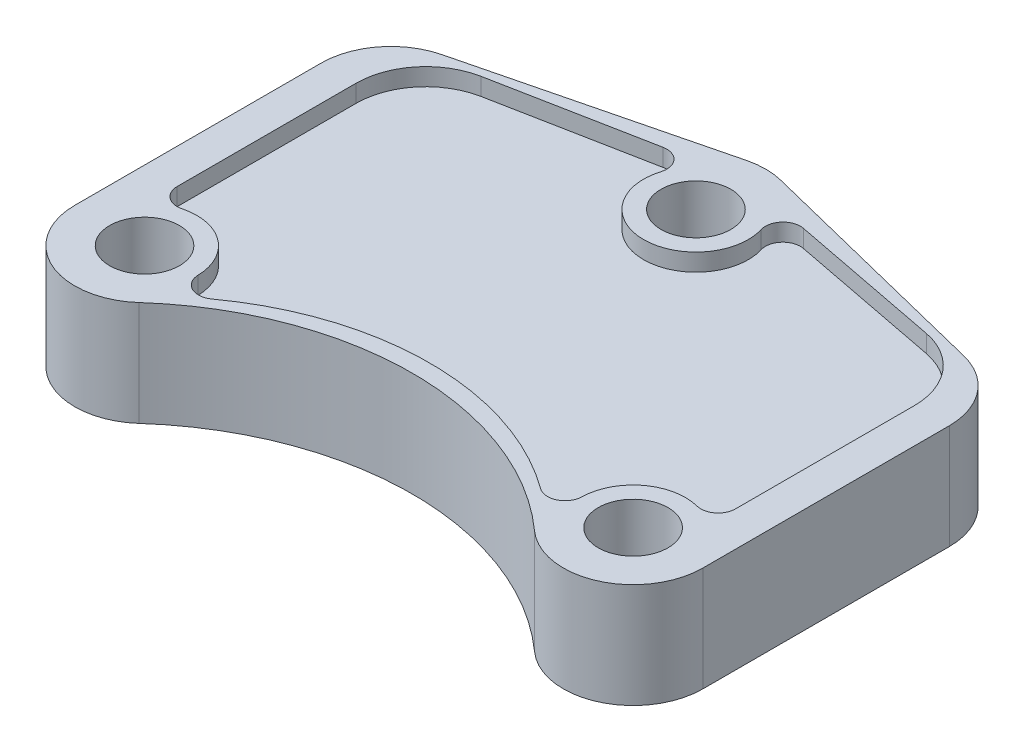
ISO-10303-21;
HEADER;
FILE_DESCRIPTION(('STEP AP214'),'2;1');
FILE_NAME('part.step','',(''),(''),'','','');
FILE_SCHEMA(('AUTOMOTIVE_DESIGN { 1 0 10303 214 1 1 1 1 }'));
ENDSEC;
DATA;
#1=APPLICATION_CONTEXT('core data for automotive mechanical design processes');
#2=APPLICATION_PROTOCOL_DEFINITION('international standard','automotive_design',2000,#1);
#3=PRODUCT_CONTEXT('',#1,'mechanical');
#4=PRODUCT('Part','Part','',(#3));
#5=PRODUCT_RELATED_PRODUCT_CATEGORY('part','',(#4));
#6=PRODUCT_DEFINITION_FORMATION('','',#4);
#7=PRODUCT_DEFINITION_CONTEXT('part definition',#1,'design');
#8=PRODUCT_DEFINITION('design','',#6,#7);
#9=PRODUCT_DEFINITION_SHAPE('','',#8);
#10=(LENGTH_UNIT() NAMED_UNIT(*) SI_UNIT(.MILLI.,.METRE.));
#11=(NAMED_UNIT(*) PLANE_ANGLE_UNIT() SI_UNIT($,.RADIAN.));
#12=(NAMED_UNIT(*) SI_UNIT($,.STERADIAN.) SOLID_ANGLE_UNIT());
#13=UNCERTAINTY_MEASURE_WITH_UNIT(LENGTH_MEASURE(1.E-05),#10,'distance_accuracy_value','');
#14=(GEOMETRIC_REPRESENTATION_CONTEXT(3) GLOBAL_UNCERTAINTY_ASSIGNED_CONTEXT((#13)) GLOBAL_UNIT_ASSIGNED_CONTEXT((#10,
#11,#12)) REPRESENTATION_CONTEXT('',''));
#15=CARTESIAN_POINT('',(0.,0.,0.));
#16=DIRECTION('',(0.,0.,1.));
#17=DIRECTION('',(1.,0.,0.));
#18=AXIS2_PLACEMENT_3D('',#15,#16,#17);
#19=CARTESIAN_POINT('',(-50.0055751114862,30.,87.5277994307735));
#20=DIRECTION('',(0.,-1.,0.));
#21=DIRECTION('',(0.,0.,-1.));
#22=AXIS2_PLACEMENT_3D('',#19,#20,#21);
#23=CYLINDRICAL_SURFACE('',#22,5.);
#24=DIRECTION('',(0.,-1.,0.));
#25=VECTOR('',#24,1.);
#26=CARTESIAN_POINT('',(-47.0640706931635,30.,91.5710100061687));
#27=LINE('',#26,#25);
#28=CARTESIAN_POINT('',(-47.0640706931635,30.,91.5710100061687));
#29=VERTEX_POINT('',#28);
#30=CARTESIAN_POINT('',(-47.0640706931635,25.,91.5710100061687));
#31=VERTEX_POINT('',#30);
#32=EDGE_CURVE('E268',#29,#31,#27,.T.);
#33=ORIENTED_EDGE('',*,*,#32,.T.);
#34=CARTESIAN_POINT('',(-50.0055751114862,25.,87.5277994307735));
#35=DIRECTION('',(0.,-1.,0.));
#36=DIRECTION('',(0.,0.,-1.));
#37=AXIS2_PLACEMENT_3D('',#34,#35,#36);
#38=CIRCLE('',#37,4.99999999999999);
#39=CARTESIAN_POINT('',(-55.0041813336146,25.,87.6458495730801));
#40=VERTEX_POINT('',#39);
#41=EDGE_CURVE('E740',#31,#40,#38,.T.);
#42=ORIENTED_EDGE('',*,*,#41,.T.);
#43=DIRECTION('',(0.,-1.,0.));
#44=VECTOR('',#43,1.);
#45=CARTESIAN_POINT('',(-55.0041813336146,30.,87.6458495730801));
#46=LINE('',#45,#44);
#47=CARTESIAN_POINT('',(-55.0041813336146,30.,87.6458495730801));
#48=VERTEX_POINT('',#47);
#49=EDGE_CURVE('E724',#48,#40,#46,.T.);
#50=ORIENTED_EDGE('',*,*,#49,.F.);
#51=CARTESIAN_POINT('',(-50.0055751114862,30.,87.5277994307735));
#52=DIRECTION('',(0.,1.,0.));
#53=DIRECTION('',(0.,0.,1.));
#54=AXIS2_PLACEMENT_3D('',#51,#52,#53);
#55=CIRCLE('',#54,5.);
#56=EDGE_CURVE('E731',#48,#29,#55,.T.);
#57=ORIENTED_EDGE('',*,*,#56,.T.);
#58=EDGE_LOOP('',(#33,#42,#50,#57));
#59=FACE_BOUND('',#58,.T.);
#60=ADVANCED_FACE('F39',(#59),#23,.F.);
#61=CARTESIAN_POINT('',(0.,30.,156.262379212493));
#62=DIRECTION('',(0.,-1.,0.));
#63=DIRECTION('',(0.,0.,-1.));
#64=AXIS2_PLACEMENT_3D('',#61,#62,#63);
#65=CYLINDRICAL_SURFACE('',#64,80.);
#66=DIRECTION('',(0.,-1.,0.));
#67=VECTOR('',#66,1.);
#68=CARTESIAN_POINT('',(47.0640706931634,30.,91.5710100061687));
#69=LINE('',#68,#67);
#70=CARTESIAN_POINT('',(47.0640706931634,30.,91.5710100061687));
#71=VERTEX_POINT('',#70);
#72=CARTESIAN_POINT('',(47.0640706931635,25.,91.5710100061687));
#73=VERTEX_POINT('',#72);
#74=EDGE_CURVE('E264',#71,#73,#69,.T.);
#75=ORIENTED_EDGE('',*,*,#74,.T.);
#76=CARTESIAN_POINT('',(0.,25.,156.262379212493));
#77=DIRECTION('',(0.,1.,0.));
#78=DIRECTION('',(0.,0.,-1.));
#79=AXIS2_PLACEMENT_3D('',#76,#77,#78);
#80=CIRCLE('',#79,80.);
#81=EDGE_CURVE('E738',#73,#31,#80,.T.);
#82=ORIENTED_EDGE('',*,*,#81,.T.);
#83=ORIENTED_EDGE('',*,*,#32,.F.);
#84=CARTESIAN_POINT('',(0.,30.,156.262379212493));
#85=DIRECTION('',(0.,-1.,0.));
#86=DIRECTION('',(0.,0.,-1.));
#87=AXIS2_PLACEMENT_3D('',#84,#85,#86);
#88=CIRCLE('',#87,80.);
#89=EDGE_CURVE('E699',#29,#71,#88,.T.);
#90=ORIENTED_EDGE('',*,*,#89,.T.);
#91=EDGE_LOOP('',(#75,#82,#83,#90));
#92=FACE_BOUND('',#91,.T.);
#93=ADVANCED_FACE('F397',(#92),#65,.T.);
#94=CARTESIAN_POINT('',(50.0055751114862,30.,87.5277994307735));
#95=DIRECTION('',(0.,-1.,0.));
#96=DIRECTION('',(0.,0.,-1.));
#97=AXIS2_PLACEMENT_3D('',#94,#95,#96);
#98=CYLINDRICAL_SURFACE('',#97,5.);
#99=DIRECTION('',(0.,-1.,0.));
#100=VECTOR('',#99,1.);
#101=CARTESIAN_POINT('',(55.0041813336146,30.,87.6458495730801));
#102=LINE('',#101,#100);
#103=CARTESIAN_POINT('',(55.0041813336146,30.,87.6458495730801));
#104=VERTEX_POINT('',#103);
#105=CARTESIAN_POINT('',(55.0041813336146,25.,87.6458495730801));
#106=VERTEX_POINT('',#105);
#107=EDGE_CURVE('E265',#104,#106,#102,.T.);
#108=ORIENTED_EDGE('',*,*,#107,.T.);
#109=CARTESIAN_POINT('',(50.0055751114862,25.,87.5277994307735));
#110=DIRECTION('',(0.,-1.,0.));
#111=DIRECTION('',(0.,0.,-1.));
#112=AXIS2_PLACEMENT_3D('',#109,#110,#111);
#113=CIRCLE('',#112,4.99999999999999);
#114=EDGE_CURVE('E684',#106,#73,#113,.T.);
#115=ORIENTED_EDGE('',*,*,#114,.T.);
#116=ORIENTED_EDGE('',*,*,#74,.F.);
#117=CARTESIAN_POINT('',(50.0055751114862,30.,87.5277994307735));
#118=DIRECTION('',(0.,1.,0.));
#119=DIRECTION('',(0.,0.,1.));
#120=AXIS2_PLACEMENT_3D('',#117,#118,#119);
#121=CIRCLE('',#120,5.);
#122=EDGE_CURVE('E683',#71,#104,#121,.T.);
#123=ORIENTED_EDGE('',*,*,#122,.T.);
#124=EDGE_LOOP('',(#108,#115,#116,#123));
#125=FACE_BOUND('',#124,.T.);
#126=ADVANCED_FACE('F407',(#125),#98,.F.);
#127=CARTESIAN_POINT('',(70.,30.,88.));
#128=DIRECTION('',(0.,-1.,0.));
#129=DIRECTION('',(0.,0.,-1.));
#130=AXIS2_PLACEMENT_3D('',#127,#128,#129);
#131=CYLINDRICAL_SURFACE('',#130,15.);
#132=DIRECTION('',(0.,-1.,0.));
#133=VECTOR('',#132,1.);
#134=CARTESIAN_POINT('',(73.75,30.,73.4763124517222));
#135=LINE('',#134,#133);
#136=CARTESIAN_POINT('',(73.75,30.,73.4763124517222));
#137=VERTEX_POINT('',#136);
#138=CARTESIAN_POINT('',(73.75,25.,73.4763124517222));
#139=VERTEX_POINT('',#138);
#140=EDGE_CURVE('E259',#137,#139,#135,.T.);
#141=ORIENTED_EDGE('',*,*,#140,.T.);
#142=CARTESIAN_POINT('',(70.,25.,88.));
#143=DIRECTION('',(0.,1.,0.));
#144=DIRECTION('',(0.,0.,-1.));
#145=AXIS2_PLACEMENT_3D('',#142,#143,#144);
#146=CIRCLE('',#145,15.);
#147=EDGE_CURVE('E689',#139,#106,#146,.T.);
#148=ORIENTED_EDGE('',*,*,#147,.T.);
#149=ORIENTED_EDGE('',*,*,#107,.F.);
#150=CARTESIAN_POINT('',(70.,30.,88.));
#151=DIRECTION('',(0.,-1.,0.));
#152=DIRECTION('',(0.,0.,-1.));
#153=AXIS2_PLACEMENT_3D('',#150,#151,#152);
#154=CIRCLE('',#153,15.);
#155=EDGE_CURVE('E686',#104,#137,#154,.T.);
#156=ORIENTED_EDGE('',*,*,#155,.T.);
#157=EDGE_LOOP('',(#141,#148,#149,#156));
#158=FACE_BOUND('',#157,.T.);
#159=ADVANCED_FACE('F567',(#158),#131,.T.);
#160=CARTESIAN_POINT('',(75.,30.,68.6350832689629));
#161=DIRECTION('',(0.,-1.,0.));
#162=DIRECTION('',(0.,0.,-1.));
#163=AXIS2_PLACEMENT_3D('',#160,#161,#162);
#164=CYLINDRICAL_SURFACE('',#163,5.00000000000002);
#165=DIRECTION('',(0.,-1.,0.));
#166=VECTOR('',#165,1.);
#167=CARTESIAN_POINT('',(80.,30.,68.6350832689629));
#168=LINE('',#167,#166);
#169=CARTESIAN_POINT('',(80.,30.,68.6350832689629));
#170=VERTEX_POINT('',#169);
#171=CARTESIAN_POINT('',(80.,25.,68.6350832689629));
#172=VERTEX_POINT('',#171);
#173=EDGE_CURVE('E258',#170,#172,#168,.T.);
#174=ORIENTED_EDGE('',*,*,#173,.T.);
#175=CARTESIAN_POINT('',(75.,25.,68.6350832689629));
#176=DIRECTION('',(0.,-1.,0.));
#177=DIRECTION('',(0.,0.,-1.));
#178=AXIS2_PLACEMENT_3D('',#175,#176,#177);
#179=CIRCLE('',#178,5.00000000000003);
#180=EDGE_CURVE('E770',#172,#139,#179,.T.);
#181=ORIENTED_EDGE('',*,*,#180,.T.);
#182=ORIENTED_EDGE('',*,*,#140,.F.);
#183=CARTESIAN_POINT('',(75.,30.,68.6350832689629));
#184=DIRECTION('',(0.,1.,0.));
#185=DIRECTION('',(0.,0.,1.));
#186=AXIS2_PLACEMENT_3D('',#183,#184,#185);
#187=CIRCLE('',#186,5.00000000000002);
#188=EDGE_CURVE('E694',#137,#170,#187,.T.);
#189=ORIENTED_EDGE('',*,*,#188,.T.);
#190=EDGE_LOOP('',(#174,#181,#182,#189));
#191=FACE_BOUND('',#190,.T.);
#192=ADVANCED_FACE('F560',(#191),#164,.F.);
#193=CARTESIAN_POINT('',(80.,30.,68.6350832689629));
#194=DIRECTION('',(-1.,0.,0.));
#195=DIRECTION('',(0.,0.,1.));
#196=AXIS2_PLACEMENT_3D('',#193,#194,#195);
#197=PLANE('',#196);
#198=DIRECTION('',(0.,-1.,0.));
#199=VECTOR('',#198,1.);
#200=CARTESIAN_POINT('',(80.,30.,17.408786158483));
#201=LINE('',#200,#199);
#202=CARTESIAN_POINT('',(80.,30.,17.408786158483));
#203=VERTEX_POINT('',#202);
#204=CARTESIAN_POINT('',(80.,25.,17.408786158483));
#205=VERTEX_POINT('',#204);
#206=EDGE_CURVE('E251',#203,#205,#201,.T.);
#207=ORIENTED_EDGE('',*,*,#206,.T.);
#208=DIRECTION('',(0.,0.,1.));
#209=VECTOR('',#208,1.);
#210=CARTESIAN_POINT('',(80.,25.,68.6350832689629));
#211=LINE('',#210,#209);
#212=EDGE_CURVE('E772',#205,#172,#211,.T.);
#213=ORIENTED_EDGE('',*,*,#212,.T.);
#214=ORIENTED_EDGE('',*,*,#173,.F.);
#215=DIRECTION('',(0.,0.,-1.));
#216=VECTOR('',#215,1.);
#217=CARTESIAN_POINT('',(80.,30.,68.6350832689629));
#218=LINE('',#217,#216);
#219=EDGE_CURVE('E700',#170,#203,#218,.T.);
#220=ORIENTED_EDGE('',*,*,#219,.T.);
#221=EDGE_LOOP('',(#207,#213,#214,#220));
#222=FACE_BOUND('',#221,.T.);
#223=ADVANCED_FACE('F547',(#222),#197,.T.);
#224=CARTESIAN_POINT('',(60.,30.,17.408786158483));
#225=DIRECTION('',(0.,-1.,0.));
#226=DIRECTION('',(0.,0.,-1.));
#227=AXIS2_PLACEMENT_3D('',#224,#225,#226);
#228=CYLINDRICAL_SURFACE('',#227,20.);
#229=DIRECTION('',(0.,-1.,0.));
#230=VECTOR('',#229,1.);
#231=CARTESIAN_POINT('',(63.8045133363284,30.,-2.22602166521872));
#232=LINE('',#231,#230);
#233=CARTESIAN_POINT('',(63.8045133363284,30.,-2.22602166521872));
#234=VERTEX_POINT('',#233);
#235=CARTESIAN_POINT('',(63.8045133363284,25.,-2.22602166521871));
#236=VERTEX_POINT('',#235);
#237=EDGE_CURVE('E249',#234,#236,#232,.T.);
#238=ORIENTED_EDGE('',*,*,#237,.T.);
#239=CARTESIAN_POINT('',(60.,25.,17.408786158483));
#240=DIRECTION('',(0.,-1.,0.));
#241=DIRECTION('',(0.,0.,-1.));
#242=AXIS2_PLACEMENT_3D('',#239,#240,#241);
#243=CIRCLE('',#242,20.);
#244=EDGE_CURVE('E771',#236,#205,#243,.T.);
#245=ORIENTED_EDGE('',*,*,#244,.T.);
#246=ORIENTED_EDGE('',*,*,#206,.F.);
#247=CARTESIAN_POINT('',(60.,30.,17.408786158483));
#248=DIRECTION('',(0.,1.,0.));
#249=DIRECTION('',(0.,0.,1.));
#250=AXIS2_PLACEMENT_3D('',#247,#248,#249);
#251=CIRCLE('',#250,20.);
#252=EDGE_CURVE('E702',#203,#234,#251,.T.);
#253=ORIENTED_EDGE('',*,*,#252,.T.);
#254=EDGE_LOOP('',(#238,#245,#246,#253));
#255=FACE_BOUND('',#254,.T.);
#256=ADVANCED_FACE('F537',(#255),#228,.F.);
#257=CARTESIAN_POINT('',(63.8045133363284,30.,-2.22602166521872));
#258=DIRECTION('',(-0.190225666816419,0.,0.981740391185087));
#259=DIRECTION('',(0.981740391185087,0.,0.190225666816419));
#260=AXIS2_PLACEMENT_3D('',#257,#258,#259);
#261=PLANE('',#260);
#262=DIRECTION('',(0.,-1.,0.));
#263=VECTOR('',#262,1.);
#264=CARTESIAN_POINT('',(20.0957491684961,30.,-10.6951942532089));
#265=LINE('',#264,#263);
#266=CARTESIAN_POINT('',(20.0957491684961,30.,-10.6951942532089));
#267=VERTEX_POINT('',#266);
#268=CARTESIAN_POINT('',(20.0957491684961,25.,-10.6951942532089));
#269=VERTEX_POINT('',#268);
#270=EDGE_CURVE('E250',#267,#269,#265,.T.);
#271=ORIENTED_EDGE('',*,*,#270,.T.);
#272=DIRECTION('',(0.981740391185088,0.,0.190225666816419));
#273=VECTOR('',#272,1.);
#274=CARTESIAN_POINT('',(63.8045133363284,25.,-2.22602166521872));
#275=LINE('',#274,#273);
#276=EDGE_CURVE('E780',#269,#236,#275,.T.);
#277=ORIENTED_EDGE('',*,*,#276,.T.);
#278=ORIENTED_EDGE('',*,*,#237,.F.);
#279=DIRECTION('',(-0.981740391185088,0.,-0.190225666816419));
#280=VECTOR('',#279,1.);
#281=CARTESIAN_POINT('',(63.8045133363284,30.,-2.22602166521872));
#282=LINE('',#281,#280);
#283=EDGE_CURVE('E706',#234,#267,#282,.T.);
#284=ORIENTED_EDGE('',*,*,#283,.T.);
#285=EDGE_LOOP('',(#271,#277,#278,#284));
#286=FACE_BOUND('',#285,.T.);
#287=ADVANCED_FACE('F529',(#286),#261,.T.);
#288=CARTESIAN_POINT('',(19.144620834414,30.,-5.78649229728347));
#289=DIRECTION('',(0.,-1.,0.));
#290=DIRECTION('',(0.,0.,-1.));
#291=AXIS2_PLACEMENT_3D('',#288,#289,#290);
#292=CYLINDRICAL_SURFACE('',#291,5.);
#293=DIRECTION('',(0.,-1.,0.));
#294=VECTOR('',#293,1.);
#295=CARTESIAN_POINT('',(14.3584656258105,30.,-4.33986922296261));
#296=LINE('',#295,#294);
#297=CARTESIAN_POINT('',(14.3584656258105,30.,-4.33986922296261));
#298=VERTEX_POINT('',#297);
#299=CARTESIAN_POINT('',(14.3584656258105,25.,-4.33986922296261));
#300=VERTEX_POINT('',#299);
#301=EDGE_CURVE('E241',#298,#300,#296,.T.);
#302=ORIENTED_EDGE('',*,*,#301,.T.);
#303=CARTESIAN_POINT('',(19.144620834414,25.,-5.78649229728347));
#304=DIRECTION('',(0.,-1.,0.));
#305=DIRECTION('',(0.,0.,-1.));
#306=AXIS2_PLACEMENT_3D('',#303,#304,#305);
#307=CIRCLE('',#306,5.);
#308=EDGE_CURVE('E778',#300,#269,#307,.T.);
#309=ORIENTED_EDGE('',*,*,#308,.T.);
#310=ORIENTED_EDGE('',*,*,#270,.F.);
#311=CARTESIAN_POINT('',(19.144620834414,30.,-5.78649229728347));
#312=DIRECTION('',(0.,1.,0.));
#313=DIRECTION('',(0.,0.,1.));
#314=AXIS2_PLACEMENT_3D('',#311,#312,#313);
#315=CIRCLE('',#314,5.);
#316=EDGE_CURVE('E708',#267,#298,#315,.T.);
#317=ORIENTED_EDGE('',*,*,#316,.T.);
#318=EDGE_LOOP('',(#302,#309,#310,#317));
#319=FACE_BOUND('',#318,.T.);
#320=ADVANCED_FACE('F523',(#319),#292,.F.);
#321=CARTESIAN_POINT('',(0.,30.,0.));
#322=DIRECTION('',(0.,-1.,0.));
#323=DIRECTION('',(0.,0.,-1.));
#324=AXIS2_PLACEMENT_3D('',#321,#322,#323);
#325=CYLINDRICAL_SURFACE('',#324,15.);
#326=DIRECTION('',(0.,-1.,0.));
#327=VECTOR('',#326,1.);
#328=CARTESIAN_POINT('',(-14.3584656258105,30.,-4.3398692229626));
#329=LINE('',#328,#327);
#330=CARTESIAN_POINT('',(-14.3584656258105,30.,-4.3398692229626));
#331=VERTEX_POINT('',#330);
#332=CARTESIAN_POINT('',(-14.3584656258105,25.,-4.3398692229626));
#333=VERTEX_POINT('',#332);
#334=EDGE_CURVE('E237',#331,#333,#329,.T.);
#335=ORIENTED_EDGE('',*,*,#334,.T.);
#336=CARTESIAN_POINT('',(0.,25.,0.));
#337=DIRECTION('',(0.,1.,0.));
#338=DIRECTION('',(0.,0.,-1.));
#339=AXIS2_PLACEMENT_3D('',#336,#337,#338);
#340=CIRCLE('',#339,15.);
#341=EDGE_CURVE('E781',#333,#300,#340,.T.);
#342=ORIENTED_EDGE('',*,*,#341,.T.);
#343=ORIENTED_EDGE('',*,*,#301,.F.);
#344=CARTESIAN_POINT('',(0.,30.,0.));
#345=DIRECTION('',(0.,-1.,0.));
#346=DIRECTION('',(0.,0.,1.));
#347=AXIS2_PLACEMENT_3D('',#344,#345,#346);
#348=CIRCLE('',#347,15.);
#349=EDGE_CURVE('E709',#298,#331,#348,.T.);
#350=ORIENTED_EDGE('',*,*,#349,.T.);
#351=EDGE_LOOP('',(#335,#342,#343,#350));
#352=FACE_BOUND('',#351,.T.);
#353=ADVANCED_FACE('F515',(#352),#325,.T.);
#354=CARTESIAN_POINT('',(-19.144620834414,30.,-5.78649229728347));
#355=DIRECTION('',(0.,-1.,0.));
#356=DIRECTION('',(0.,0.,-1.));
#357=AXIS2_PLACEMENT_3D('',#354,#355,#356);
#358=CYLINDRICAL_SURFACE('',#357,5.);
#359=DIRECTION('',(0.,-1.,0.));
#360=VECTOR('',#359,1.);
#361=CARTESIAN_POINT('',(-20.0957491684961,30.,-10.6951942532089));
#362=LINE('',#361,#360);
#363=CARTESIAN_POINT('',(-20.0957491684961,30.,-10.6951942532089));
#364=VERTEX_POINT('',#363);
#365=CARTESIAN_POINT('',(-20.0957491684961,25.,-10.6951942532089));
#366=VERTEX_POINT('',#365);
#367=EDGE_CURVE('E232',#364,#366,#362,.T.);
#368=ORIENTED_EDGE('',*,*,#367,.T.);
#369=CARTESIAN_POINT('',(-19.144620834414,25.,-5.78649229728347));
#370=DIRECTION('',(0.,-1.,0.));
#371=DIRECTION('',(0.,0.,-1.));
#372=AXIS2_PLACEMENT_3D('',#369,#370,#371);
#373=CIRCLE('',#372,5.);
#374=EDGE_CURVE('E216',#366,#333,#373,.T.);
#375=ORIENTED_EDGE('',*,*,#374,.T.);
#376=ORIENTED_EDGE('',*,*,#334,.F.);
#377=CARTESIAN_POINT('',(-19.144620834414,30.,-5.78649229728347));
#378=DIRECTION('',(0.,1.,0.));
#379=DIRECTION('',(0.,0.,-1.));
#380=AXIS2_PLACEMENT_3D('',#377,#378,#379);
#381=CIRCLE('',#380,5.);
#382=EDGE_CURVE('E715',#331,#364,#381,.T.);
#383=ORIENTED_EDGE('',*,*,#382,.T.);
#384=EDGE_LOOP('',(#368,#375,#376,#383));
#385=FACE_BOUND('',#384,.T.);
#386=ADVANCED_FACE('F501',(#385),#358,.F.);
#387=CARTESIAN_POINT('',(-63.8045133363284,30.,-2.22602166521872));
#388=DIRECTION('',(0.190225666816419,0.,0.981740391185087));
#389=DIRECTION('',(0.981740391185087,0.,-0.190225666816419));
#390=AXIS2_PLACEMENT_3D('',#387,#388,#389);
#391=PLANE('',#390);
#392=DIRECTION('',(0.,-1.,0.));
#393=VECTOR('',#392,1.);
#394=CARTESIAN_POINT('',(-63.8045133363284,30.,-2.22602166521871));
#395=LINE('',#394,#393);
#396=CARTESIAN_POINT('',(-63.8045133363284,30.,-2.22602166521871));
#397=VERTEX_POINT('',#396);
#398=CARTESIAN_POINT('',(-63.8045133363284,25.,-2.22602166521871));
#399=VERTEX_POINT('',#398);
#400=EDGE_CURVE('E227',#397,#399,#395,.T.);
#401=ORIENTED_EDGE('',*,*,#400,.T.);
#402=DIRECTION('',(0.981740391185087,0.,-0.190225666816419));
#403=VECTOR('',#402,1.);
#404=CARTESIAN_POINT('',(-20.0957491684961,25.,-10.6951942532089));
#405=LINE('',#404,#403);
#406=EDGE_CURVE('E209',#399,#366,#405,.T.);
#407=ORIENTED_EDGE('',*,*,#406,.T.);
#408=ORIENTED_EDGE('',*,*,#367,.F.);
#409=DIRECTION('',(-0.981740391185088,0.,0.190225666816419));
#410=VECTOR('',#409,1.);
#411=CARTESIAN_POINT('',(-63.8045133363284,30.,-2.22602166521872));
#412=LINE('',#411,#410);
#413=EDGE_CURVE('E231',#364,#397,#412,.T.);
#414=ORIENTED_EDGE('',*,*,#413,.T.);
#415=EDGE_LOOP('',(#401,#407,#408,#414));
#416=FACE_BOUND('',#415,.T.);
#417=ADVANCED_FACE('F233',(#416),#391,.T.);
#418=CARTESIAN_POINT('',(-60.,30.,17.408786158483));
#419=DIRECTION('',(0.,-1.,0.));
#420=DIRECTION('',(0.,0.,-1.));
#421=AXIS2_PLACEMENT_3D('',#418,#419,#420);
#422=CYLINDRICAL_SURFACE('',#421,20.);
#423=DIRECTION('',(0.,-1.,0.));
#424=VECTOR('',#423,1.);
#425=CARTESIAN_POINT('',(-80.,30.,17.408786158483));
#426=LINE('',#425,#424);
#427=CARTESIAN_POINT('',(-80.,30.,17.408786158483));
#428=VERTEX_POINT('',#427);
#429=CARTESIAN_POINT('',(-80.,25.,17.408786158483));
#430=VERTEX_POINT('',#429);
#431=EDGE_CURVE('E226',#428,#430,#426,.T.);
#432=ORIENTED_EDGE('',*,*,#431,.T.);
#433=CARTESIAN_POINT('',(-60.,25.,17.408786158483));
#434=DIRECTION('',(0.,-1.,0.));
#435=DIRECTION('',(0.,0.,-1.));
#436=AXIS2_PLACEMENT_3D('',#433,#434,#435);
#437=CIRCLE('',#436,20.);
#438=EDGE_CURVE('E213',#430,#399,#437,.T.);
#439=ORIENTED_EDGE('',*,*,#438,.T.);
#440=ORIENTED_EDGE('',*,*,#400,.F.);
#441=CARTESIAN_POINT('',(-60.,30.,17.408786158483));
#442=DIRECTION('',(0.,1.,0.));
#443=DIRECTION('',(0.,0.,-1.));
#444=AXIS2_PLACEMENT_3D('',#441,#442,#443);
#445=CIRCLE('',#444,20.);
#446=EDGE_CURVE('E714',#397,#428,#445,.T.);
#447=ORIENTED_EDGE('',*,*,#446,.T.);
#448=EDGE_LOOP('',(#432,#439,#440,#447));
#449=FACE_BOUND('',#448,.T.);
#450=ADVANCED_FACE('F223',(#449),#422,.F.);
#451=CARTESIAN_POINT('',(-80.,30.,68.6350832689629));
#452=DIRECTION('',(1.,0.,0.));
#453=DIRECTION('',(0.,0.,-1.));
#454=AXIS2_PLACEMENT_3D('',#451,#452,#453);
#455=PLANE('',#454);
#456=DIRECTION('',(0.,-1.,0.));
#457=VECTOR('',#456,1.);
#458=CARTESIAN_POINT('',(-80.,30.,68.6350832689629));
#459=LINE('',#458,#457);
#460=CARTESIAN_POINT('',(-80.,30.,68.6350832689629));
#461=VERTEX_POINT('',#460);
#462=CARTESIAN_POINT('',(-80.,25.,68.6350832689629));
#463=VERTEX_POINT('',#462);
#464=EDGE_CURVE('E236',#461,#463,#459,.T.);
#465=ORIENTED_EDGE('',*,*,#464,.T.);
#466=DIRECTION('',(0.,0.,-1.));
#467=VECTOR('',#466,1.);
#468=CARTESIAN_POINT('',(-80.,25.,17.408786158483));
#469=LINE('',#468,#467);
#470=EDGE_CURVE('E726',#463,#430,#469,.T.);
#471=ORIENTED_EDGE('',*,*,#470,.T.);
#472=ORIENTED_EDGE('',*,*,#431,.F.);
#473=DIRECTION('',(0.,0.,1.));
#474=VECTOR('',#473,1.);
#475=CARTESIAN_POINT('',(-80.,30.,68.6350832689629));
#476=LINE('',#475,#474);
#477=EDGE_CURVE('E720',#428,#461,#476,.T.);
#478=ORIENTED_EDGE('',*,*,#477,.T.);
#479=EDGE_LOOP('',(#465,#471,#472,#478));
#480=FACE_BOUND('',#479,.T.);
#481=ADVANCED_FACE('F477',(#480),#455,.T.);
#482=CARTESIAN_POINT('',(-75.,30.,68.6350832689629));
#483=DIRECTION('',(0.,-1.,0.));
#484=DIRECTION('',(0.,0.,-1.));
#485=AXIS2_PLACEMENT_3D('',#482,#483,#484);
#486=CYLINDRICAL_SURFACE('',#485,5.00000000000001);
#487=DIRECTION('',(0.,-1.,0.));
#488=VECTOR('',#487,1.);
#489=CARTESIAN_POINT('',(-73.75,30.,73.4763124517222));
#490=LINE('',#489,#488);
#491=CARTESIAN_POINT('',(-73.75,30.,73.4763124517222));
#492=VERTEX_POINT('',#491);
#493=CARTESIAN_POINT('',(-73.75,25.,73.4763124517222));
#494=VERTEX_POINT('',#493);
#495=EDGE_CURVE('E62',#492,#494,#490,.T.);
#496=ORIENTED_EDGE('',*,*,#495,.T.);
#497=CARTESIAN_POINT('',(-75.,25.,68.6350832689629));
#498=DIRECTION('',(0.,-1.,0.));
#499=DIRECTION('',(0.,0.,-1.));
#500=AXIS2_PLACEMENT_3D('',#497,#498,#499);
#501=CIRCLE('',#500,5.00000000000001);
#502=EDGE_CURVE('E53',#494,#463,#501,.T.);
#503=ORIENTED_EDGE('',*,*,#502,.T.);
#504=ORIENTED_EDGE('',*,*,#464,.F.);
#505=CARTESIAN_POINT('',(-75.,30.,68.6350832689629));
#506=DIRECTION('',(0.,1.,0.));
#507=DIRECTION('',(0.,0.,-1.));
#508=AXIS2_PLACEMENT_3D('',#505,#506,#507);
#509=CIRCLE('',#508,5.00000000000001);
#510=EDGE_CURVE('E716',#461,#492,#509,.T.);
#511=ORIENTED_EDGE('',*,*,#510,.T.);
#512=EDGE_LOOP('',(#496,#503,#504,#511));
#513=FACE_BOUND('',#512,.T.);
#514=ADVANCED_FACE('F472',(#513),#486,.F.);
#515=CARTESIAN_POINT('',(-70.,30.,88.));
#516=DIRECTION('',(0.,-1.,0.));
#517=DIRECTION('',(0.,0.,-1.));
#518=AXIS2_PLACEMENT_3D('',#515,#516,#517);
#519=CYLINDRICAL_SURFACE('',#518,15.);
#520=ORIENTED_EDGE('',*,*,#49,.T.);
#521=CARTESIAN_POINT('',(-70.,25.,88.));
#522=DIRECTION('',(0.,1.,0.));
#523=DIRECTION('',(0.,0.,-1.));
#524=AXIS2_PLACEMENT_3D('',#521,#522,#523);
#525=CIRCLE('',#524,15.);
#526=EDGE_CURVE('E736',#40,#494,#525,.T.);
#527=ORIENTED_EDGE('',*,*,#526,.T.);
#528=ORIENTED_EDGE('',*,*,#495,.F.);
#529=CARTESIAN_POINT('',(-70.,30.,88.));
#530=DIRECTION('',(0.,-1.,0.));
#531=DIRECTION('',(0.,0.,1.));
#532=AXIS2_PLACEMENT_3D('',#529,#530,#531);
#533=CIRCLE('',#532,15.);
#534=EDGE_CURVE('E722',#492,#48,#533,.T.);
#535=ORIENTED_EDGE('',*,*,#534,.T.);
#536=EDGE_LOOP('',(#520,#527,#528,#535));
#537=FACE_BOUND('',#536,.T.);
#538=ADVANCED_FACE('F411',(#537),#519,.T.);
#539=CARTESIAN_POINT('',(-70.,30.,88.));
#540=DIRECTION('',(0.,1.,0.));
#541=DIRECTION('',(0.,0.,1.));
#542=AXIS2_PLACEMENT_3D('',#539,#540,#541);
#543=PLANE('',#542);
#544=CARTESIAN_POINT('',(-70.,30.,88.));
#545=DIRECTION('',(0.,1.,0.));
#546=DIRECTION('',(0.,0.,1.));
#547=AXIS2_PLACEMENT_3D('',#544,#545,#546);
#548=CIRCLE('',#547,10.);
#549=CARTESIAN_POINT('',(-70.,30.,98.));
#550=VERTEX_POINT('',#549);
#551=EDGE_CURVE('E752',#550,#550,#548,.T.);
#552=ORIENTED_EDGE('',*,*,#551,.F.);
#553=EDGE_LOOP('',(#552));
#554=FACE_BOUND('',#553,.T.);
#555=ORIENTED_EDGE('',*,*,#89,.F.);
#556=ORIENTED_EDGE('',*,*,#56,.F.);
#557=ORIENTED_EDGE('',*,*,#534,.F.);
#558=ORIENTED_EDGE('',*,*,#510,.F.);
#559=ORIENTED_EDGE('',*,*,#477,.F.);
#560=ORIENTED_EDGE('',*,*,#446,.F.);
#561=ORIENTED_EDGE('',*,*,#413,.F.);
#562=ORIENTED_EDGE('',*,*,#382,.F.);
#563=ORIENTED_EDGE('',*,*,#349,.F.);
#564=ORIENTED_EDGE('',*,*,#316,.F.);
#565=ORIENTED_EDGE('',*,*,#283,.F.);
#566=ORIENTED_EDGE('',*,*,#252,.F.);
#567=ORIENTED_EDGE('',*,*,#219,.F.);
#568=ORIENTED_EDGE('',*,*,#188,.F.);
#569=ORIENTED_EDGE('',*,*,#155,.F.);
#570=ORIENTED_EDGE('',*,*,#122,.F.);
#571=EDGE_LOOP('',(#555,#556,#557,#558,#559,#560,#561,#562,#563,#564,#565,#566,#567,#568,#569,#570));
#572=FACE_BOUND('',#571,.T.);
#573=CARTESIAN_POINT('',(-70.,30.,88.));
#574=DIRECTION('',(0.,1.,0.));
#575=DIRECTION('',(0.,0.,1.));
#576=AXIS2_PLACEMENT_3D('',#573,#574,#575);
#577=CIRCLE('',#576,20.);
#578=CARTESIAN_POINT('',(-90.,30.,88.));
#579=VERTEX_POINT('',#578);
#580=CARTESIAN_POINT('',(-56.6666666666667,30.,102.907119849999));
#581=VERTEX_POINT('',#580);
#582=EDGE_CURVE('E275',#579,#581,#577,.T.);
#583=ORIENTED_EDGE('',*,*,#582,.T.);
#584=CARTESIAN_POINT('',(0.,30.,166.262379212493));
#585=DIRECTION('',(0.,-1.,0.));
#586=DIRECTION('',(0.,0.,-1.));
#587=AXIS2_PLACEMENT_3D('',#584,#585,#586);
#588=CIRCLE('',#587,85.);
#589=CARTESIAN_POINT('',(56.6666666666667,30.,102.907119849999));
#590=VERTEX_POINT('',#589);
#591=EDGE_CURVE('E274',#581,#590,#588,.T.);
#592=ORIENTED_EDGE('',*,*,#591,.T.);
#593=CARTESIAN_POINT('',(70.,30.,88.));
#594=DIRECTION('',(0.,1.,0.));
#595=DIRECTION('',(0.,0.,-1.));
#596=AXIS2_PLACEMENT_3D('',#593,#594,#595);
#597=CIRCLE('',#596,20.);
#598=CARTESIAN_POINT('',(90.,30.,88.));
#599=VERTEX_POINT('',#598);
#600=EDGE_CURVE('E279',#590,#599,#597,.T.);
#601=ORIENTED_EDGE('',*,*,#600,.T.);
#602=DIRECTION('',(0.,0.,-1.));
#603=VECTOR('',#602,1.);
#604=CARTESIAN_POINT('',(90.,30.,88.));
#605=LINE('',#604,#603);
#606=CARTESIAN_POINT('',(90.0000000000001,30.,17.408786158483));
#607=VERTEX_POINT('',#606);
#608=EDGE_CURVE('E278',#599,#607,#605,.T.);
#609=ORIENTED_EDGE('',*,*,#608,.T.);
#610=CARTESIAN_POINT('',(70.,30.,17.408786158483));
#611=DIRECTION('',(0.,1.,0.));
#612=DIRECTION('',(0.,0.,1.));
#613=AXIS2_PLACEMENT_3D('',#610,#611,#612);
#614=CIRCLE('',#613,20.);
#615=CARTESIAN_POINT('',(74.8269058261252,30.,-2.));
#616=VERTEX_POINT('',#615);
#617=EDGE_CURVE('E285',#607,#616,#614,.T.);
#618=ORIENTED_EDGE('',*,*,#617,.T.);
#619=DIRECTION('',(-0.970439307924148,0.,-0.241345291306253));
#620=VECTOR('',#619,1.);
#621=CARTESIAN_POINT('',(74.8269058261252,30.,-2.));
#622=LINE('',#621,#620);
#623=CARTESIAN_POINT('',(4.82690582612508,30.,-19.408786158483));
#624=VERTEX_POINT('',#623);
#625=EDGE_CURVE('E281',#616,#624,#622,.T.);
#626=ORIENTED_EDGE('',*,*,#625,.T.);
#627=CARTESIAN_POINT('',(0.,30.,0.));
#628=DIRECTION('',(0.,1.,0.));
#629=DIRECTION('',(0.,0.,1.));
#630=AXIS2_PLACEMENT_3D('',#627,#628,#629);
#631=CIRCLE('',#630,20.);
#632=CARTESIAN_POINT('',(-4.82690582612508,30.,-19.408786158483));
#633=VERTEX_POINT('',#632);
#634=EDGE_CURVE('E288',#624,#633,#631,.T.);
#635=ORIENTED_EDGE('',*,*,#634,.T.);
#636=DIRECTION('',(-0.970439307924148,0.,0.241345291306253));
#637=VECTOR('',#636,1.);
#638=CARTESIAN_POINT('',(-74.8269058261252,30.,-2.));
#639=LINE('',#638,#637);
#640=CARTESIAN_POINT('',(-74.8269058261252,30.,-1.99999999999996));
#641=VERTEX_POINT('',#640);
#642=EDGE_CURVE('E286',#633,#641,#639,.T.);
#643=ORIENTED_EDGE('',*,*,#642,.T.);
#644=CARTESIAN_POINT('',(-70.,30.,17.408786158483));
#645=DIRECTION('',(0.,1.,0.));
#646=DIRECTION('',(0.,0.,-1.));
#647=AXIS2_PLACEMENT_3D('',#644,#645,#646);
#648=CIRCLE('',#647,20.);
#649=CARTESIAN_POINT('',(-90.,30.,17.408786158483));
#650=VERTEX_POINT('',#649);
#651=EDGE_CURVE('E289',#641,#650,#648,.T.);
#652=ORIENTED_EDGE('',*,*,#651,.T.);
#653=DIRECTION('',(0.,0.,1.));
#654=VECTOR('',#653,1.);
#655=CARTESIAN_POINT('',(-90.,30.,88.));
#656=LINE('',#655,#654);
#657=EDGE_CURVE('E295',#650,#579,#656,.T.);
#658=ORIENTED_EDGE('',*,*,#657,.T.);
#659=EDGE_LOOP('',(#583,#592,#601,#609,#618,#626,#635,#643,#652,#658));
#660=FACE_BOUND('',#659,.T.);
#661=CARTESIAN_POINT('',(0.,30.,0.));
#662=DIRECTION('',(0.,1.,0.));
#663=DIRECTION('',(0.,0.,1.));
#664=AXIS2_PLACEMENT_3D('',#661,#662,#663);
#665=CIRCLE('',#664,10.);
#666=CARTESIAN_POINT('',(0.,30.,10.));
#667=VERTEX_POINT('',#666);
#668=EDGE_CURVE('E761',#667,#667,#665,.T.);
#669=ORIENTED_EDGE('',*,*,#668,.F.);
#670=EDGE_LOOP('',(#669));
#671=FACE_BOUND('',#670,.T.);
#672=CARTESIAN_POINT('',(70.,30.,88.));
#673=DIRECTION('',(0.,1.,0.));
#674=DIRECTION('',(0.,0.,-1.));
#675=AXIS2_PLACEMENT_3D('',#672,#673,#674);
#676=CIRCLE('',#675,10.);
#677=CARTESIAN_POINT('',(70.,30.,78.));
#678=VERTEX_POINT('',#677);
#679=EDGE_CURVE('E750',#678,#678,#676,.T.);
#680=ORIENTED_EDGE('',*,*,#679,.F.);
#681=EDGE_LOOP('',(#680));
#682=FACE_BOUND('',#681,.T.);
#683=ADVANCED_FACE('F363',(#554,#572,#660,#671,#682),#543,.T.);
#684=CARTESIAN_POINT('',(-70.,0.,88.));
#685=DIRECTION('',(0.,1.,0.));
#686=DIRECTION('',(0.,0.,1.));
#687=AXIS2_PLACEMENT_3D('',#684,#685,#686);
#688=PLANE('',#687);
#689=CARTESIAN_POINT('',(-70.,0.,88.));
#690=DIRECTION('',(0.,1.,0.));
#691=DIRECTION('',(0.,0.,1.));
#692=AXIS2_PLACEMENT_3D('',#689,#690,#691);
#693=CIRCLE('',#692,20.);
#694=CARTESIAN_POINT('',(-90.,0.,88.));
#695=VERTEX_POINT('',#694);
#696=CARTESIAN_POINT('',(-56.6666666666667,0.,102.907119849999));
#697=VERTEX_POINT('',#696);
#698=EDGE_CURVE('E271',#695,#697,#693,.T.);
#699=ORIENTED_EDGE('',*,*,#698,.F.);
#700=DIRECTION('',(0.,0.,1.));
#701=VECTOR('',#700,1.);
#702=CARTESIAN_POINT('',(-90.,0.,88.));
#703=LINE('',#702,#701);
#704=CARTESIAN_POINT('',(-90.,0.,17.408786158483));
#705=VERTEX_POINT('',#704);
#706=EDGE_CURVE('E277',#705,#695,#703,.T.);
#707=ORIENTED_EDGE('',*,*,#706,.F.);
#708=CARTESIAN_POINT('',(-70.,0.,17.408786158483));
#709=DIRECTION('',(0.,1.,0.));
#710=DIRECTION('',(0.,0.,-1.));
#711=AXIS2_PLACEMENT_3D('',#708,#709,#710);
#712=CIRCLE('',#711,20.);
#713=CARTESIAN_POINT('',(-74.8269058261252,0.,-1.99999999999996));
#714=VERTEX_POINT('',#713);
#715=EDGE_CURVE('E313',#714,#705,#712,.T.);
#716=ORIENTED_EDGE('',*,*,#715,.F.);
#717=DIRECTION('',(-0.970439307924148,0.,0.241345291306253));
#718=VECTOR('',#717,1.);
#719=CARTESIAN_POINT('',(-74.8269058261252,0.,-2.));
#720=LINE('',#719,#718);
#721=CARTESIAN_POINT('',(-4.82690582612508,0.,-19.408786158483));
#722=VERTEX_POINT('',#721);
#723=EDGE_CURVE('E310',#722,#714,#720,.T.);
#724=ORIENTED_EDGE('',*,*,#723,.F.);
#725=CARTESIAN_POINT('',(0.,0.,0.));
#726=DIRECTION('',(0.,1.,0.));
#727=DIRECTION('',(0.,0.,1.));
#728=AXIS2_PLACEMENT_3D('',#725,#726,#727);
#729=CIRCLE('',#728,20.);
#730=CARTESIAN_POINT('',(4.82690582612508,0.,-19.408786158483));
#731=VERTEX_POINT('',#730);
#732=EDGE_CURVE('E307',#731,#722,#729,.T.);
#733=ORIENTED_EDGE('',*,*,#732,.F.);
#734=DIRECTION('',(-0.970439307924148,0.,-0.241345291306253));
#735=VECTOR('',#734,1.);
#736=CARTESIAN_POINT('',(74.8269058261252,0.,-2.));
#737=LINE('',#736,#735);
#738=CARTESIAN_POINT('',(74.8269058261252,0.,-2.));
#739=VERTEX_POINT('',#738);
#740=EDGE_CURVE('E304',#739,#731,#737,.T.);
#741=ORIENTED_EDGE('',*,*,#740,.F.);
#742=CARTESIAN_POINT('',(70.,0.,17.408786158483));
#743=DIRECTION('',(0.,1.,0.));
#744=DIRECTION('',(0.,0.,1.));
#745=AXIS2_PLACEMENT_3D('',#742,#743,#744);
#746=CIRCLE('',#745,20.);
#747=CARTESIAN_POINT('',(90.0000000000001,0.,17.408786158483));
#748=VERTEX_POINT('',#747);
#749=EDGE_CURVE('E301',#748,#739,#746,.T.);
#750=ORIENTED_EDGE('',*,*,#749,.F.);
#751=DIRECTION('',(0.,0.,-1.));
#752=VECTOR('',#751,1.);
#753=CARTESIAN_POINT('',(90.,0.,88.));
#754=LINE('',#753,#752);
#755=CARTESIAN_POINT('',(90.,0.,88.));
#756=VERTEX_POINT('',#755);
#757=EDGE_CURVE('E303',#756,#748,#754,.T.);
#758=ORIENTED_EDGE('',*,*,#757,.F.);
#759=CARTESIAN_POINT('',(70.,0.,88.));
#760=DIRECTION('',(0.,1.,0.));
#761=DIRECTION('',(0.,0.,-1.));
#762=AXIS2_PLACEMENT_3D('',#759,#760,#761);
#763=CIRCLE('',#762,20.);
#764=CARTESIAN_POINT('',(56.6666666666667,0.,102.907119849999));
#765=VERTEX_POINT('',#764);
#766=EDGE_CURVE('E296',#765,#756,#763,.T.);
#767=ORIENTED_EDGE('',*,*,#766,.F.);
#768=CARTESIAN_POINT('',(0.,0.,166.262379212493));
#769=DIRECTION('',(0.,-1.,0.));
#770=DIRECTION('',(0.,0.,-1.));
#771=AXIS2_PLACEMENT_3D('',#768,#769,#770);
#772=CIRCLE('',#771,85.);
#773=EDGE_CURVE('E300',#697,#765,#772,.T.);
#774=ORIENTED_EDGE('',*,*,#773,.F.);
#775=EDGE_LOOP('',(#699,#707,#716,#724,#733,#741,#750,#758,#767,#774));
#776=FACE_BOUND('',#775,.T.);
#777=CARTESIAN_POINT('',(0.,0.,0.));
#778=DIRECTION('',(0.,1.,0.));
#779=DIRECTION('',(0.,0.,1.));
#780=AXIS2_PLACEMENT_3D('',#777,#778,#779);
#781=CIRCLE('',#780,10.);
#782=CARTESIAN_POINT('',(0.,0.,10.));
#783=VERTEX_POINT('',#782);
#784=EDGE_CURVE('E758',#783,#783,#781,.T.);
#785=ORIENTED_EDGE('',*,*,#784,.T.);
#786=EDGE_LOOP('',(#785));
#787=FACE_BOUND('',#786,.T.);
#788=CARTESIAN_POINT('',(-70.,0.,88.));
#789=DIRECTION('',(0.,1.,0.));
#790=DIRECTION('',(0.,0.,1.));
#791=AXIS2_PLACEMENT_3D('',#788,#789,#790);
#792=CIRCLE('',#791,10.);
#793=CARTESIAN_POINT('',(-70.,0.,98.));
#794=VERTEX_POINT('',#793);
#795=EDGE_CURVE('E755',#794,#794,#792,.T.);
#796=ORIENTED_EDGE('',*,*,#795,.T.);
#797=EDGE_LOOP('',(#796));
#798=FACE_BOUND('',#797,.T.);
#799=CARTESIAN_POINT('',(70.,0.,88.));
#800=DIRECTION('',(0.,1.,0.));
#801=DIRECTION('',(0.,0.,-1.));
#802=AXIS2_PLACEMENT_3D('',#799,#800,#801);
#803=CIRCLE('',#802,10.);
#804=CARTESIAN_POINT('',(70.,0.,78.));
#805=VERTEX_POINT('',#804);
#806=EDGE_CURVE('E746',#805,#805,#803,.T.);
#807=ORIENTED_EDGE('',*,*,#806,.T.);
#808=EDGE_LOOP('',(#807));
#809=FACE_BOUND('',#808,.T.);
#810=ADVANCED_FACE('F350',(#776,#787,#798,#809),#688,.F.);
#811=CARTESIAN_POINT('',(-70.,30.,88.));
#812=DIRECTION('',(0.,-1.,0.));
#813=DIRECTION('',(0.,0.,-1.));
#814=AXIS2_PLACEMENT_3D('',#811,#812,#813);
#815=CYLINDRICAL_SURFACE('',#814,20.);
#816=ORIENTED_EDGE('',*,*,#698,.T.);
#817=DIRECTION('',(0.,-1.,0.));
#818=VECTOR('',#817,1.);
#819=CARTESIAN_POINT('',(-56.6666666666667,30.,102.907119849999));
#820=LINE('',#819,#818);
#821=EDGE_CURVE('E11',#581,#697,#820,.T.);
#822=ORIENTED_EDGE('',*,*,#821,.F.);
#823=ORIENTED_EDGE('',*,*,#582,.F.);
#824=DIRECTION('',(0.,-1.,0.));
#825=VECTOR('',#824,1.);
#826=CARTESIAN_POINT('',(-90.,30.,88.));
#827=LINE('',#826,#825);
#828=EDGE_CURVE('E294',#579,#695,#827,.T.);
#829=ORIENTED_EDGE('',*,*,#828,.T.);
#830=EDGE_LOOP('',(#816,#822,#823,#829));
#831=FACE_BOUND('',#830,.T.);
#832=ADVANCED_FACE('F41',(#831),#815,.T.);
#833=CARTESIAN_POINT('',(0.,30.,166.262379212493));
#834=DIRECTION('',(0.,-1.,0.));
#835=DIRECTION('',(0.,0.,-1.));
#836=AXIS2_PLACEMENT_3D('',#833,#834,#835);
#837=CYLINDRICAL_SURFACE('',#836,85.);
#838=ORIENTED_EDGE('',*,*,#773,.T.);
#839=DIRECTION('',(0.,-1.,0.));
#840=VECTOR('',#839,1.);
#841=CARTESIAN_POINT('',(56.6666666666667,30.,102.907119849999));
#842=LINE('',#841,#840);
#843=EDGE_CURVE('E50',#590,#765,#842,.T.);
#844=ORIENTED_EDGE('',*,*,#843,.F.);
#845=ORIENTED_EDGE('',*,*,#591,.F.);
#846=ORIENTED_EDGE('',*,*,#821,.T.);
#847=EDGE_LOOP('',(#838,#844,#845,#846));
#848=FACE_BOUND('',#847,.T.);
#849=ADVANCED_FACE('F368',(#848),#837,.F.);
#850=CARTESIAN_POINT('',(70.,30.,88.));
#851=DIRECTION('',(0.,-1.,0.));
#852=DIRECTION('',(0.,0.,-1.));
#853=AXIS2_PLACEMENT_3D('',#850,#851,#852);
#854=CYLINDRICAL_SURFACE('',#853,20.);
#855=ORIENTED_EDGE('',*,*,#766,.T.);
#856=DIRECTION('',(0.,-1.,0.));
#857=VECTOR('',#856,1.);
#858=CARTESIAN_POINT('',(90.,30.,88.));
#859=LINE('',#858,#857);
#860=EDGE_CURVE('E331',#599,#756,#859,.T.);
#861=ORIENTED_EDGE('',*,*,#860,.F.);
#862=ORIENTED_EDGE('',*,*,#600,.F.);
#863=ORIENTED_EDGE('',*,*,#843,.T.);
#864=EDGE_LOOP('',(#855,#861,#862,#863));
#865=FACE_BOUND('',#864,.T.);
#866=ADVANCED_FACE('F343',(#865),#854,.T.);
#867=CARTESIAN_POINT('',(90.,30.,88.));
#868=DIRECTION('',(-1.,0.,0.));
#869=DIRECTION('',(0.,0.,1.));
#870=AXIS2_PLACEMENT_3D('',#867,#868,#869);
#871=PLANE('',#870);
#872=ORIENTED_EDGE('',*,*,#757,.T.);
#873=DIRECTION('',(0.,-1.,0.));
#874=VECTOR('',#873,1.);
#875=CARTESIAN_POINT('',(90.0000000000001,30.,17.408786158483));
#876=LINE('',#875,#874);
#877=EDGE_CURVE('E332',#607,#748,#876,.T.);
#878=ORIENTED_EDGE('',*,*,#877,.F.);
#879=ORIENTED_EDGE('',*,*,#608,.F.);
#880=ORIENTED_EDGE('',*,*,#860,.T.);
#881=EDGE_LOOP('',(#872,#878,#879,#880));
#882=FACE_BOUND('',#881,.T.);
#883=ADVANCED_FACE('F354',(#882),#871,.F.);
#884=CARTESIAN_POINT('',(70.,30.,17.408786158483));
#885=DIRECTION('',(0.,-1.,0.));
#886=DIRECTION('',(0.,0.,-1.));
#887=AXIS2_PLACEMENT_3D('',#884,#885,#886);
#888=CYLINDRICAL_SURFACE('',#887,20.);
#889=ORIENTED_EDGE('',*,*,#749,.T.);
#890=DIRECTION('',(0.,-1.,0.));
#891=VECTOR('',#890,1.);
#892=CARTESIAN_POINT('',(74.8269058261252,30.,-2.));
#893=LINE('',#892,#891);
#894=EDGE_CURVE('E327',#616,#739,#893,.T.);
#895=ORIENTED_EDGE('',*,*,#894,.F.);
#896=ORIENTED_EDGE('',*,*,#617,.F.);
#897=ORIENTED_EDGE('',*,*,#877,.T.);
#898=EDGE_LOOP('',(#889,#895,#896,#897));
#899=FACE_BOUND('',#898,.T.);
#900=ADVANCED_FACE('F360',(#899),#888,.T.);
#901=CARTESIAN_POINT('',(74.8269058261252,30.,-2.));
#902=DIRECTION('',(-0.241345291306253,0.,0.970439307924148));
#903=DIRECTION('',(0.970439307924148,0.,0.241345291306253));
#904=AXIS2_PLACEMENT_3D('',#901,#902,#903);
#905=PLANE('',#904);
#906=ORIENTED_EDGE('',*,*,#740,.T.);
#907=DIRECTION('',(0.,-1.,0.));
#908=VECTOR('',#907,1.);
#909=CARTESIAN_POINT('',(4.82690582612508,30.,-19.408786158483));
#910=LINE('',#909,#908);
#911=EDGE_CURVE('E324',#624,#731,#910,.T.);
#912=ORIENTED_EDGE('',*,*,#911,.F.);
#913=ORIENTED_EDGE('',*,*,#625,.F.);
#914=ORIENTED_EDGE('',*,*,#894,.T.);
#915=EDGE_LOOP('',(#906,#912,#913,#914));
#916=FACE_BOUND('',#915,.T.);
#917=ADVANCED_FACE('F386',(#916),#905,.F.);
#918=CARTESIAN_POINT('',(0.,30.,0.));
#919=DIRECTION('',(0.,-1.,0.));
#920=DIRECTION('',(0.,0.,-1.));
#921=AXIS2_PLACEMENT_3D('',#918,#919,#920);
#922=CYLINDRICAL_SURFACE('',#921,20.);
#923=ORIENTED_EDGE('',*,*,#732,.T.);
#924=DIRECTION('',(0.,-1.,0.));
#925=VECTOR('',#924,1.);
#926=CARTESIAN_POINT('',(-4.82690582612508,30.,-19.408786158483));
#927=LINE('',#926,#925);
#928=EDGE_CURVE('E325',#633,#722,#927,.T.);
#929=ORIENTED_EDGE('',*,*,#928,.F.);
#930=ORIENTED_EDGE('',*,*,#634,.F.);
#931=ORIENTED_EDGE('',*,*,#911,.T.);
#932=EDGE_LOOP('',(#923,#929,#930,#931));
#933=FACE_BOUND('',#932,.T.);
#934=ADVANCED_FACE('F387',(#933),#922,.T.);
#935=CARTESIAN_POINT('',(-74.8269058261252,30.,-2.));
#936=DIRECTION('',(0.241345291306253,0.,0.970439307924148));
#937=DIRECTION('',(0.970439307924148,0.,-0.241345291306253));
#938=AXIS2_PLACEMENT_3D('',#935,#936,#937);
#939=PLANE('',#938);
#940=ORIENTED_EDGE('',*,*,#723,.T.);
#941=DIRECTION('',(0.,-1.,0.));
#942=VECTOR('',#941,1.);
#943=CARTESIAN_POINT('',(-74.8269058261252,30.,-1.99999999999996));
#944=LINE('',#943,#942);
#945=EDGE_CURVE('E317',#641,#714,#944,.T.);
#946=ORIENTED_EDGE('',*,*,#945,.F.);
#947=ORIENTED_EDGE('',*,*,#642,.F.);
#948=ORIENTED_EDGE('',*,*,#928,.T.);
#949=EDGE_LOOP('',(#940,#946,#947,#948));
#950=FACE_BOUND('',#949,.T.);
#951=ADVANCED_FACE('F385',(#950),#939,.F.);
#952=CARTESIAN_POINT('',(-70.,30.,17.408786158483));
#953=DIRECTION('',(0.,-1.,0.));
#954=DIRECTION('',(0.,0.,-1.));
#955=AXIS2_PLACEMENT_3D('',#952,#953,#954);
#956=CYLINDRICAL_SURFACE('',#955,20.);
#957=ORIENTED_EDGE('',*,*,#715,.T.);
#958=DIRECTION('',(0.,-1.,0.));
#959=VECTOR('',#958,1.);
#960=CARTESIAN_POINT('',(-90.,30.,17.408786158483));
#961=LINE('',#960,#959);
#962=EDGE_CURVE('E316',#650,#705,#961,.T.);
#963=ORIENTED_EDGE('',*,*,#962,.F.);
#964=ORIENTED_EDGE('',*,*,#651,.F.);
#965=ORIENTED_EDGE('',*,*,#945,.T.);
#966=EDGE_LOOP('',(#957,#963,#964,#965));
#967=FACE_BOUND('',#966,.T.);
#968=ADVANCED_FACE('F378',(#967),#956,.T.);
#969=CARTESIAN_POINT('',(-90.,30.,88.));
#970=DIRECTION('',(1.,0.,0.));
#971=DIRECTION('',(0.,0.,-1.));
#972=AXIS2_PLACEMENT_3D('',#969,#970,#971);
#973=PLANE('',#972);
#974=ORIENTED_EDGE('',*,*,#706,.T.);
#975=ORIENTED_EDGE('',*,*,#828,.F.);
#976=ORIENTED_EDGE('',*,*,#657,.F.);
#977=ORIENTED_EDGE('',*,*,#962,.T.);
#978=EDGE_LOOP('',(#974,#975,#976,#977));
#979=FACE_BOUND('',#978,.T.);
#980=ADVANCED_FACE('F373',(#979),#973,.F.);
#981=CARTESIAN_POINT('',(0.,30.,0.));
#982=DIRECTION('',(0.,-1.,0.));
#983=DIRECTION('',(0.,0.,-1.));
#984=AXIS2_PLACEMENT_3D('',#981,#982,#983);
#985=CYLINDRICAL_SURFACE('',#984,10.);
#986=ORIENTED_EDGE('',*,*,#668,.T.);
#987=EDGE_LOOP('',(#986));
#988=FACE_BOUND('',#987,.T.);
#989=ORIENTED_EDGE('',*,*,#784,.F.);
#990=EDGE_LOOP('',(#989));
#991=FACE_BOUND('',#990,.T.);
#992=ADVANCED_FACE('F420',(#988,#991),#985,.F.);
#993=CARTESIAN_POINT('',(-70.,30.,88.));
#994=DIRECTION('',(0.,-1.,0.));
#995=DIRECTION('',(0.,0.,-1.));
#996=AXIS2_PLACEMENT_3D('',#993,#994,#995);
#997=CYLINDRICAL_SURFACE('',#996,10.);
#998=ORIENTED_EDGE('',*,*,#551,.T.);
#999=EDGE_LOOP('',(#998));
#1000=FACE_BOUND('',#999,.T.);
#1001=ORIENTED_EDGE('',*,*,#795,.F.);
#1002=EDGE_LOOP('',(#1001));
#1003=FACE_BOUND('',#1002,.T.);
#1004=ADVANCED_FACE('F441',(#1000,#1003),#997,.F.);
#1005=CARTESIAN_POINT('',(70.,30.,88.));
#1006=DIRECTION('',(0.,-1.,0.));
#1007=DIRECTION('',(0.,0.,-1.));
#1008=AXIS2_PLACEMENT_3D('',#1005,#1006,#1007);
#1009=CYLINDRICAL_SURFACE('',#1008,10.);
#1010=ORIENTED_EDGE('',*,*,#679,.T.);
#1011=EDGE_LOOP('',(#1010));
#1012=FACE_BOUND('',#1011,.T.);
#1013=ORIENTED_EDGE('',*,*,#806,.F.);
#1014=EDGE_LOOP('',(#1013));
#1015=FACE_BOUND('',#1014,.T.);
#1016=ADVANCED_FACE('F455',(#1012,#1015),#1009,.F.);
#1017=CARTESIAN_POINT('',(-60.,25.,17.408786158483));
#1018=DIRECTION('',(0.,-1.,0.));
#1019=DIRECTION('',(0.,0.,-1.));
#1020=AXIS2_PLACEMENT_3D('',#1017,#1018,#1019);
#1021=PLANE('',#1020);
#1022=ORIENTED_EDGE('',*,*,#438,.F.);
#1023=ORIENTED_EDGE('',*,*,#470,.F.);
#1024=ORIENTED_EDGE('',*,*,#502,.F.);
#1025=ORIENTED_EDGE('',*,*,#526,.F.);
#1026=ORIENTED_EDGE('',*,*,#41,.F.);
#1027=ORIENTED_EDGE('',*,*,#81,.F.);
#1028=ORIENTED_EDGE('',*,*,#114,.F.);
#1029=ORIENTED_EDGE('',*,*,#147,.F.);
#1030=ORIENTED_EDGE('',*,*,#180,.F.);
#1031=ORIENTED_EDGE('',*,*,#212,.F.);
#1032=ORIENTED_EDGE('',*,*,#244,.F.);
#1033=ORIENTED_EDGE('',*,*,#276,.F.);
#1034=ORIENTED_EDGE('',*,*,#308,.F.);
#1035=ORIENTED_EDGE('',*,*,#341,.F.);
#1036=ORIENTED_EDGE('',*,*,#374,.F.);
#1037=ORIENTED_EDGE('',*,*,#406,.F.);
#1038=EDGE_LOOP('',(#1022,#1023,#1024,#1025,#1026,#1027,#1028,#1029,#1030,#1031,#1032,#1033,
#1034,#1035,#1036,#1037));
#1039=FACE_BOUND('',#1038,.T.);
#1040=ADVANCED_FACE('F215',(#1039),#1021,.F.);
#1041=CLOSED_SHELL('',(#60,#93,#126,#159,#192,#223,#256,#287,#320,#353,#386,#417,#450,#481,#514,
#538,#683,#810,#832,#849,#866,#883,#900,#917,#934,#951,#968,#980,#992,#1004,#1016,#1040));
#1042=MANIFOLD_SOLID_BREP('B2',#1041);
#1043=ADVANCED_BREP_SHAPE_REPRESENTATION('',(#18,#1042),#14);
#1044=SHAPE_DEFINITION_REPRESENTATION(#9,#1043);
ENDSEC;
END-ISO-10303-21;
